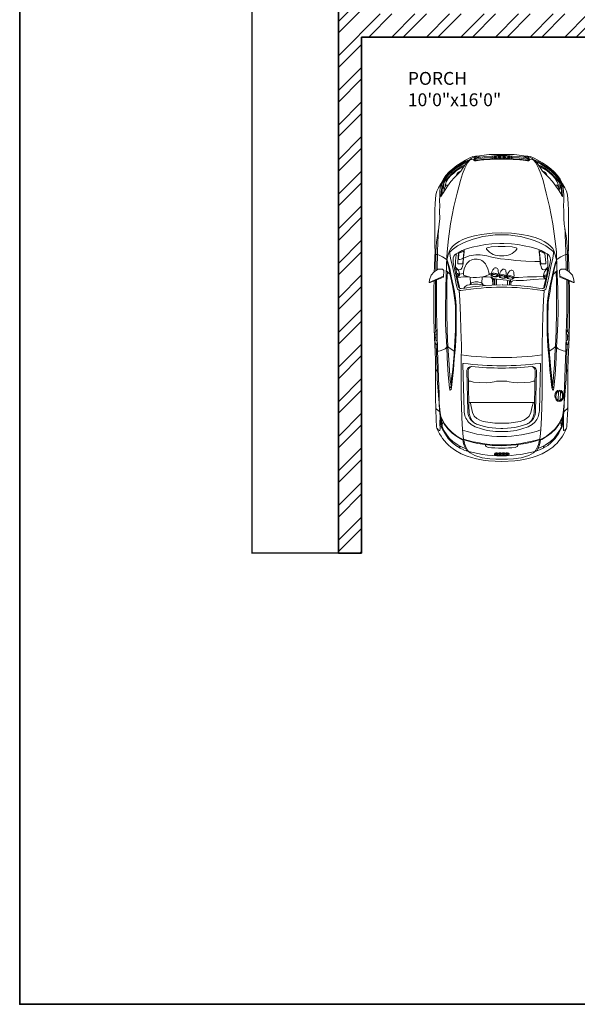
# Model space of a CAD drawing. Units: inches. Extents: x 1152 to 2588, y 1459 to 2618.
# Tile 1 of 17: x 1152 to 1369, y 1459 to 1843. Entities that reach past the tile are written whole.
import ezdxf

# ---------------------------------------------------------------- set-up
doc = ezdxf.new("R2010")
doc.units = ezdxf.units.IN
for name, color, linetype, lineweight in [('A-ANNO-DIMS', 2, 'Continuous', 18), ('A-ANNO-TTLB', 7, 'Continuous', 35), ('A-AREA-IDEN', 7, 'Continuous', 18), ('A-WALL', 7, 'Continuous', 35), ('A-WALL-PATT', 8, 'Continuous', 13), ('AUDI', 7, 'Continuous', 13)]:
    doc.layers.add(name, color=color, linetype=linetype, lineweight=lineweight)
doc.styles.get("Standard").update_dxf_attribs({"font": 'arial.ttf'})
doc.dimstyles.get("Standard").update_dxf_attribs({"dimtxt": 0.18, "dimasz": 0.18, "dimexe": 0.18, "dimexo": 0.0625, "dimgap": 0.09, "dimtad": 0, "dimtih": 1, "dimtoh": 1, "dimdec": 4, "dimzin": 0, "dimdsep": 46, "dimtxsty": 'Standard', "dimcen": 0.09, "dimadec": 0, "dimazin": 0, "dimtfac": 1, "dimtdec": 4, "dimtofl": 0, "dimtmove": 0, "dimatfit": 3, "dimfxl": 1, "dimtolj": 1, "dimtzin": 0, "dimarcsym": 0})

# ---------------------------------------------------------------- blocks, each defined once
blk = doc.blocks.new('*D71')
at = {"layer": 'A-ANNO-DIMS', "color": 0, "lineweight": -2, "transparency": 16777216}
for p, q in [((1276.35, 2240.05), (1242.64, 2240.05)), ((1242.82, 2239.87), (1242.82, 1937.73)), ((1242.82, 1635.23), (1242.82, 1937.36)), ((1276.35, 1635.05), (1242.64, 1635.05))]:
    blk.add_line(p, q, dxfattribs=at)
at = {"layer": 'A-ANNO-DIMS', "color": 0, "transparency": 16777216}
for points in [[(1242.79, 2239.87), (1242.85, 2239.87), (1242.82, 2240.05)], [(1242.79, 1635.23), (1242.85, 1635.23), (1242.82, 1635.05)]]:
    blk.add_solid(points, dxfattribs=at)
at = {"layer": 'Defpoints', "color": 0, "transparency": 16777216}
for p in [(1242.82, 2240.05), (1276.42, 2240.05), (1276.42, 1635.05)]:
    blk.add_point(p, dxfattribs=at)
at = {"layer": 'A-ANNO-DIMS', "color": 0, "transparency": 16777216, "insert": (1242.82, 1937.55), "char_height": 0.18, "attachment_point": 5}
blk.add_mtext('\\A1;605', dxfattribs=at)

msp = doc.modelspace()

# ---------------------------------------------------------------- hatches: boundary and pattern name
at = {"layer": 'A-WALL-PATT'}
h = msp.add_hatch(dxfattribs=at)
h.set_pattern_fill('ANSI32', color=256)
h.paths.add_polyline_path([(1408.9272, 2240.0458), (1276.4165, 2240.0458), (1276.4165, 2192.7491), (1285.4165, 2192.7491), (1285.4165, 2231.0458), (1369.4165, 2231.0458), (1369.4165, 2084.0458), (1526.9165, 2084.0458), (1526.9165, 2096.3728), (1524.6665, 2096.3728), (1522.4165, 2096.3728), (1522.4165, 2093.0458), (1378.4165, 2093.0458), (1378.4165, 2231.0458), (1408.9272, 2231.0458)])
h.paths.add_polyline_path([(1736.4165, 2240.0458), (1468.9272, 2240.0458), (1468.9272, 2231.0458), (1522.4165, 2231.0458), (1522.4165, 2127.3313), (1526.9165, 2127.3313), (1526.9165, 2231.0458), (1574.9165, 2231.0458), (1574.9165, 2188.0458), (1579.4165, 2188.0458), (1579.4165, 2231.0458), (1727.4165, 2231.0458), (1727.4165, 2183.9728), (1736.4165, 2183.9728)])
h.paths.add_polyline_path([(1285.4165, 2156.7491), (1276.4165, 2156.7491), (1276.4165, 2084.0458), (1285.4165, 2084.0458)], flags=17)
h.paths.add_polyline_path([(1285.4165, 2043.5458), (1445.4165, 2043.5458), (1445.4165, 1943.6503), (1454.4165, 1943.6503), (1454.4165, 2048.0458), (1276.4165, 2048.0458), (1276.4165, 2019.2077), (1280.9165, 2019.2077), (1285.4165, 2019.2077)])
h.paths.add_polyline_path([(1285.4165, 1959.2077), (1276.4165, 1959.2077), (1276.4165, 1891.1319), (1280.9165, 1891.1319), (1285.4165, 1891.1319), (1285.4165, 1901.0458), (1376.8505, 1901.0458), (1376.8505, 1903.2958), (1376.8505, 1905.5458), (1285.4165, 1905.5458)])
h.paths.add_polyline_path([(1518.4165, 1905.5458), (1399.2832, 1905.5458), (1399.2832, 1903.2958), (1399.2832, 1901.0458), (1405.4165, 1901.0458), (1405.4165, 1884.8579), (1409.9165, 1884.8579), (1409.9165, 1901.0458), (1513.9165, 1901.0458), (1513.9165, 1869.1706), (1518.4165, 1869.1706)])
h.paths.add_polyline_path([(1520.5229, 1845.0458), (1518.4165, 1845.0458), (1518.4165, 1849.2927), (1516.1665, 1849.2927), (1513.9165, 1849.2927), (1513.9165, 1845.0458), (1409.9165, 1845.0458), (1409.9165, 1860.8579), (1405.4165, 1860.8579), (1405.4165, 1845.0458), (1285.4165, 1845.0458), (1285.4165, 1867.1319), (1276.4165, 1867.1319), (1276.4165, 1635.0458), (1285.4165, 1635.0458), (1285.4165, 1836.0458), (1405.4165, 1836.0458), (1405.4165, 1635.0458), (1414.4165, 1635.0458), (1424.7277, 1635.0458), (1424.7277, 1639.5458), (1424.7277, 1644.0458), (1414.4165, 1644.0458), (1414.4165, 1836.0458), (1414.4165, 1840.5831), (1520.5229, 1840.5831)])
h.paths.add_polyline_path([(1579.4165, 1840.5458), (1583.4035, 1840.5458), (1583.4035, 1845.0458), (1579.4165, 1845.0458), (1570.4165, 1845.0458), (1570.4165, 1840.5831), (1570.4165, 1644.0458), (1548.2359, 1644.0458), (1548.2359, 1635.0458), (1611.2801, 1635.0458), (1611.2801, 1639.5458), (1611.2801, 1644.0458), (1579.4165, 1644.0458)])
h.paths.add_polyline_path([(1488.2359, 1644.0458), (1472.0663, 1644.0458), (1472.0663, 1635.0458), (1488.2359, 1635.0458), (1488.2359, 1639.5458)], flags=17)
h.paths.add_polyline_path([(1736.4165, 1701.1863), (1727.4165, 1701.1863), (1727.4165, 1644.0458), (1671.2801, 1644.0458), (1671.2801, 1635.0458), (1736.4165, 1635.0458)])
h.paths.add_polyline_path([(1736.4165, 2147.9728), (1727.4165, 2147.9728), (1727.4165, 2093.0458), (1579.4165, 2093.0458), (1574.9165, 2093.0458), (1574.9165, 1971.6501), (1579.4165, 1971.6501), (1579.4165, 2084.0458), (1727.4165, 2084.0458), (1727.4165, 2054.3847), (1736.4165, 2054.3847)])
h.paths.add_polyline_path([(1736.4165, 1994.3847), (1727.4165, 1994.3847), (1727.4165, 1911.3562), (1736.4165, 1911.3562)])
h.paths.add_polyline_path([(1736.4165, 1875.3562), (1727.4165, 1875.3562), (1727.4165, 1845.0458), (1617.1767, 1845.0458), (1617.1767, 1842.7958), (1617.1767, 1840.5458), (1618.9165, 1840.5458), (1618.9165, 1788.5458), (1618.9165, 1784.0458), (1627.8699, 1784.0458), (1627.8699, 1788.5458), (1623.4165, 1788.5458), (1623.4165, 1840.5458), (1727.4165, 1840.5458), (1727.4165, 1828.7619), (1736.4165, 1828.7619)])
h.paths.add_polyline_path([(1727.4165, 1938.0458), (1579.4165, 1938.0458), (1579.4165, 1942.7722), (1574.9165, 1942.7722), (1574.9165, 1929.0458), (1727.4165, 1929.0458)])

# ---------------------------------------------------------------- linework, layer by layer
at = {"layer": 'A-ANNO-TTLB'}
msp.add_lwpolyline([(1152.3215, 2617.6685), (2587.6987, 2617.6685), (2587.6987, 1459.3148), (1152.3215, 1459.3148)], close=True, dxfattribs=at)
at = {"layer": 'A-WALL'}
for p, q in [((1276.4165, 2048.0458), (1276.4165, 1635.0458)), ((1285.4165, 1836.0458), (1405.4165, 1836.0458)), ((1285.4165, 1836.0458), (1285.4165, 1635.0458)), ((1276.4165, 1635.0458), (1285.4165, 1635.0458))]:
    msp.add_line(p, q, dxfattribs=at)
at = {"layer": 'AUDI'}
for p, q in [((1336.2642, 1788.9641), (1336.2642, 1789.3086)), ((1338.3183, 1788.6147), (1338.3183, 1788.9592)), ((1341.9032, 1788.6147), (1341.9032, 1788.9592)), ((1343.9573, 1788.9641), (1343.9573, 1789.3086)), ((1324.4285, 1743.7759), (1323.5691, 1743.6789)), ((1325.138, 1743.8957), (1324.4285, 1743.7759)), ((1336.3949, 1741.7306), (1336.6785, 1741.7306)), ((1337.9694, 1741.854), (1337.9694, 1739.4675)), ((1342.3316, 1741.2324), (1342.3316, 1739.4615)), ((1352.8881, 1693.669), (1327.1848, 1693.669)), ((1323.4445, 1676.9323), (1323.6352, 1676.0919)), ((1323.8057, 1676.7406), (1323.7884, 1676.0051)), ((1356.2671, 1676.7406), (1356.2844, 1676.0051)), ((1356.6283, 1676.9323), (1356.4377, 1676.0919)), ((1337.1736, 1673.7524), (1337.1736, 1673.4961)), ((1338.7024, 1674.0125), (1338.7024, 1673.7561)), ((1341.3704, 1674.0125), (1341.3704, 1673.7561)), ((1342.8992, 1673.7524), (1342.8992, 1673.4961))]:
    msp.add_line(p, q, dxfattribs=at)
for points in [[(1330.6512, 1789.6915), (1329.8192, 1789.6915), (1328.8394, 1789.5322), (1327.6534, 1789.0235), (1325.9309, 1788.1193), (1324.2084, 1787.0173), (1322.5424, 1786.0283), (1320.9611, 1784.785), (1319.5492, 1783.5135), (1318.3056, 1782.1062), (1317.333, 1780.676), (1316.3603, 1778.928), (1315.4075, 1777.2992), (1314.7921, 1776.0477), (1314.4348, 1774.6573), (1314.1379, 1771.2484), (1314.0524, 1768.6062), (1314.0524, 1754.0739), (1314.0871, 1753.1593), (1314.1886, 1752.2446), (1313.9855, 1750.7203), (1313.8332, 1746.452), (1313.7887, 1744.543)], [(1314.0607, 1751.2847), (1314.4242, 1751.3887), (1315.0168, 1751.3145), (1315.6464, 1751.0551), (1317.0168, 1750.4251), (1318.4242, 1749.4985), (1318.7575, 1749.1279), (1319.1139, 1748.3445), (1319.7923, 1745.7397), (1320.518, 1742.235), (1321.3068, 1738.7145), (1321.6223, 1736.9622), (1321.7643, 1735.9518), (1322.0424, 1734.2928), (1322.3397, 1731.511), (1322.2994, 1728.038), (1322.3397, 1723.9593), (1322.2695, 1720.8795), (1322.0184, 1715.5567), (1321.5846, 1710.5309), (1321.2422, 1706.3732), (1320.8752, 1703.0862), (1320.4735, 1699.5786), (1320.2909, 1698.7748), (1319.9623, 1698.5556), (1319.8194, 1698.6697), (1319.6702, 1699.3959), (1319.1956, 1704.438), (1318.8305, 1711.0878), (1318.6844, 1715.3261), (1318.4288, 1719.674), (1318.2098, 1724.168), (1318.1002, 1729.6852), (1318.2165, 1737.9788), (1318.3917, 1743.4135), (1318.5669, 1747.2119), (1318.6399, 1750.1589), (1318.7567, 1752.3795), (1319.3407, 1757.522), (1320.1582, 1763.2488), (1321.443, 1770.0275), (1322.6693, 1775.2284), (1323.9541, 1780.1371), (1324.7793, 1782.7893), (1325.7137, 1785.0099), (1326.7064, 1787.0552), (1327.2327, 1787.7697), (1327.775, 1788.3646)], [(1329.2496, 1788.5039), (1328.2354, 1788.3227), (1327.2308, 1787.9457), (1326.603, 1787.5688), (1326.4356, 1787.3594), (1325.7241, 1786.1029), (1325.0126, 1785.1815), (1324.0918, 1783.8412), (1322.878, 1782.501), (1321.6642, 1781.412), (1320.1993, 1779.7786), (1318.9018, 1777.9357), (1317.981, 1776.5117), (1317.0602, 1775.1295), (1316.5998, 1774.1663), (1316.4324, 1773.9987), (1316.3487, 1773.9987), (1316.5161, 1775.7997), (1316.6835, 1777.5169), (1316.7254, 1778.6477), (1316.8091, 1779.1922), (1317.1858, 1779.9461), (1318.4414, 1781.789), (1319.6133, 1783.0035), (1320.9108, 1784.3438), (1322.2502, 1785.3071), (1324.1755, 1786.6055), (1325.8496, 1787.5269), (1327.3564, 1788.2808), (1327.775, 1788.3646), (1328.1516, 1788.7834), (1328.9469, 1789.1603), (1329.6584, 1789.4116), (1330.6167, 1789.67)], [(1326.4846, 1787.4206), (1324.8452, 1786.6055), (1323.3384, 1785.6422), (1321.9153, 1784.6788), (1320.7015, 1783.6737), (1319.5715, 1782.5847), (1318.7763, 1781.7471), (1318.0647, 1780.7419), (1317.3113, 1779.6948), (1317.0184, 1779.1503), (1316.782, 1779.016)], [(1340.0364, 1790.3413), (1340.0364, 1790.3413), (1337.6279, 1790.3413), (1337.6279, 1790.3413), (1335.1392, 1790.2551), (1332.1678, 1789.8744), (1330.6512, 1789.6915), (1330.3045, 1789.4748), (1329.878, 1789.215), (1329.3216, 1788.6539), (1329.1358, 1788.2666), (1329.2287, 1787.9292), (1329.5041, 1787.8441), (1330.0536, 1787.861), (1331.6987, 1788.1229), (1333.0121, 1788.2705), (1333.96, 1788.3095), (1335.5087, 1788.4025), (1338.0487, 1788.4335), (1339.9621, 1788.4335), (1340.0364, 1788.4335)], [(1331.9134, 1789.8437), (1331.2008, 1789.5527), (1330.4775, 1789.1907), (1329.8747, 1788.6679), (1329.5532, 1788.2658), (1329.4326, 1788.0044), (1329.4222, 1787.8694)], [(1329.6272, 1788.3584), (1330.854, 1788.5815), (1333.1941, 1788.9717), (1335.7508, 1789.1885), (1336.2748, 1789.2409)], [(1329.823, 1787.926), (1330.5526, 1788.0588), (1332.8927, 1788.4489), (1335.4494, 1788.6657), (1336.3669, 1788.7575)], [(1349.848, 1788.9716), (1349.1183, 1789.1043), (1346.7783, 1789.4945), (1344.2216, 1789.7112), (1342.0549, 1789.928), (1340.6682, 1789.9714), (1340.1107, 1789.9714), (1339.5533, 1789.9714), (1338.1666, 1789.928), (1335.9999, 1789.7112), (1333.4432, 1789.4945), (1331.1031, 1789.1043), (1330.1854, 1788.9374)], [(1340.0364, 1790.3413), (1340.0364, 1790.3413), (1342.4449, 1790.3413), (1342.4449, 1790.3413), (1344.9337, 1790.2551), (1347.905, 1789.8744), (1349.4217, 1789.6915), (1349.7683, 1789.4748), (1350.1949, 1789.215), (1350.7513, 1788.6539), (1350.937, 1788.2666), (1350.8441, 1787.9292), (1350.5688, 1787.8441), (1350.0192, 1787.861), (1348.3742, 1788.1229), (1347.0608, 1788.2705), (1346.1128, 1788.3095), (1344.5641, 1788.4025), (1342.0241, 1788.4335), (1340.1107, 1788.4335), (1340.0364, 1788.4335)], [(1340.1107, 1788.9905), (1340.1107, 1788.646)], [(1350.2499, 1787.926), (1349.5202, 1788.0588), (1347.1802, 1788.4489), (1344.6235, 1788.6657), (1343.8401, 1788.7441)], [(1350.4456, 1788.3584), (1349.2188, 1788.5815), (1346.8788, 1788.9717), (1344.3221, 1789.1885), (1343.9573, 1789.225)], [(1348.1595, 1789.8437), (1348.872, 1789.5527), (1349.5954, 1789.1907), (1350.1982, 1788.6679), (1350.5197, 1788.2658), (1350.6402, 1788.0044), (1350.6506, 1787.8694)], [(1349.4217, 1789.6915), (1350.2537, 1789.6915), (1351.2335, 1789.5322), (1352.4194, 1789.0235), (1354.1419, 1788.1193), (1355.8644, 1787.0173), (1357.5304, 1786.0283), (1359.1117, 1784.785), (1360.5236, 1783.5135), (1361.7672, 1782.1062), (1362.7399, 1780.676), (1363.7125, 1778.928), (1364.6653, 1777.2992), (1365.2807, 1776.0477), (1365.638, 1774.6573), (1365.935, 1771.2484), (1366.0204, 1768.6062), (1366.0204, 1754.0739), (1365.9858, 1753.1593), (1365.8842, 1752.2446), (1366.0873, 1750.7203), (1366.2396, 1746.452), (1366.2841, 1744.543)], [(1350.8232, 1788.5039), (1351.8375, 1788.3227), (1352.842, 1787.9457), (1353.4698, 1787.5688), (1353.6372, 1787.3594), (1354.3487, 1786.1029), (1355.0603, 1785.1815), (1355.9811, 1783.8412), (1357.1949, 1782.501), (1358.4086, 1781.412), (1359.8735, 1779.7786), (1361.171, 1777.9357), (1362.0918, 1776.5117), (1363.0126, 1775.1295), (1363.473, 1774.1663), (1363.6404, 1773.9987), (1363.7242, 1773.9987), (1363.5567, 1775.7997), (1363.3893, 1777.5169), (1363.3475, 1778.6477), (1363.2637, 1779.1922), (1362.8871, 1779.9461), (1361.6314, 1781.789), (1360.4595, 1783.0035), (1359.162, 1784.3438), (1357.8227, 1785.3071), (1355.8974, 1786.6055), (1354.2232, 1787.5269), (1352.7164, 1788.2808), (1352.2979, 1788.3646), (1351.9212, 1788.7834), (1351.126, 1789.1603), (1350.4144, 1789.4116), (1349.4562, 1789.67)], [(1366.0121, 1751.2847), (1365.6486, 1751.3887), (1365.056, 1751.3145), (1364.4264, 1751.0551), (1363.0561, 1750.4251), (1361.6487, 1749.4985), (1361.3153, 1749.1279), (1360.9589, 1748.3445), (1360.2805, 1745.7397), (1359.5548, 1742.235), (1358.766, 1738.7145), (1358.4505, 1736.9622), (1358.3085, 1735.9518), (1358.0305, 1734.2928), (1357.7331, 1731.511), (1357.7734, 1728.038), (1357.7331, 1723.9593), (1357.8033, 1720.8795), (1358.0545, 1715.5567), (1358.4882, 1710.5309), (1358.8306, 1706.3732), (1359.1977, 1703.0862), (1359.5993, 1699.5786), (1359.7819, 1698.7748), (1360.1105, 1698.5556), (1360.2534, 1698.6697), (1360.4026, 1699.3959), (1360.8772, 1704.438), (1361.2424, 1711.0878), (1361.3884, 1715.3261), (1361.644, 1719.674), (1361.8631, 1724.168), (1361.9726, 1729.6852), (1361.8563, 1737.9788), (1361.6811, 1743.4135), (1361.5059, 1747.2119), (1361.4329, 1750.1589), (1361.3161, 1752.3795), (1360.7321, 1757.522), (1359.9146, 1763.2488), (1358.6298, 1770.0275), (1357.4035, 1775.2284), (1356.1188, 1780.1371), (1355.2935, 1782.7893), (1354.3592, 1785.0099), (1353.3664, 1787.0552), (1352.8401, 1787.7697), (1352.2979, 1788.3646)], [(1353.5883, 1787.4206), (1355.2277, 1786.6055), (1356.7344, 1785.6422), (1358.1575, 1784.6788), (1359.3713, 1783.6737), (1360.5014, 1782.5847), (1361.2966, 1781.7471), (1362.0081, 1780.7419), (1362.7615, 1779.6948), (1363.0545, 1779.1503), (1363.2908, 1779.016)], [(1316.7036, 1774.3833), (1316.8091, 1775.9672), (1317.0184, 1777.6425), (1317.3113, 1778.8571), (1318.0229, 1779.988), (1319.3204, 1781.5376), (1320.4923, 1782.7941), (1321.4968, 1783.7156), (1322.292, 1784.3019), (1323.4221, 1785.0558), (1324.5522, 1785.7259), (1325.3055, 1786.061), (1325.8452, 1786.3168)], [(1317.9646, 1777.6641), (1318.1066, 1778.5639), (1318.4414, 1779.6948), (1319.1529, 1780.9094), (1320.3249, 1782.2497), (1321.3294, 1783.0873), (1322.4594, 1784.0506), (1323.7151, 1784.8464), (1324.8452, 1785.5584), (1325.4828, 1785.7904)], [(1363.3693, 1774.3833), (1363.2637, 1775.9672), (1363.0545, 1777.6425), (1362.7615, 1778.8571), (1362.05, 1779.988), (1360.7525, 1781.5376), (1359.5806, 1782.7941), (1358.5761, 1783.7156), (1357.7808, 1784.3019), (1356.6507, 1785.0558), (1355.5207, 1785.7259), (1354.7673, 1786.061), (1354.2276, 1786.3168)], [(1362.1082, 1777.6641), (1361.9662, 1778.5639), (1361.6314, 1779.6948), (1360.9199, 1780.9094), (1359.748, 1782.2497), (1358.7435, 1783.0873), (1357.6134, 1784.0506), (1356.3578, 1784.8464), (1355.2277, 1785.5584), (1354.59, 1785.7904)], [(1316.7942, 1779.0952), (1316.432, 1778.3862), (1316.1541, 1777.6679), (1316.0383, 1777.1813), (1315.9225, 1776.1154), (1315.8993, 1774.192), (1315.8762, 1772.2456), (1315.9457, 1770.4844), (1315.8762, 1768.0745), (1315.8993, 1765.4328), (1315.7372, 1763.2315), (1315.3667, 1760.8679), (1315.2761, 1758.8381), (1315.1279, 1755.7249), (1315.0909, 1752.6117), (1315.0168, 1750.9069), (1314.9057, 1746.6818), (1314.9057, 1745.3425)], [(1317.4377, 1779.058), (1317.395, 1777.3075), (1317.4355, 1776.9924), (1317.677, 1776.8005)], [(1317.5625, 1775.8834), (1317.7299, 1777.2237), (1318.0647, 1777.8519), (1318.3996, 1778.3546), (1318.9018, 1778.3964), (1319.2262, 1778.3964)], [(1362.5104, 1775.8834), (1362.3429, 1777.2237), (1362.0081, 1777.8519), (1361.6733, 1778.3546), (1361.171, 1778.3964), (1360.8467, 1778.3964)], [(1362.6351, 1779.058), (1362.6778, 1777.3075), (1362.6373, 1776.9924), (1362.3958, 1776.8005)], [(1363.2787, 1779.0952), (1363.6409, 1778.3862), (1363.9188, 1777.6679), (1364.0345, 1777.1813), (1364.1503, 1776.1154), (1364.1735, 1774.192), (1364.1966, 1772.2456), (1364.1272, 1770.4844), (1364.1966, 1768.0745), (1364.1735, 1765.4328), (1364.3356, 1763.2315), (1364.7061, 1760.8679), (1364.7968, 1758.8381), (1364.9449, 1755.7249), (1364.982, 1752.6117), (1365.056, 1750.9069), (1365.1671, 1746.6818), (1365.1671, 1745.3425)], [(1315.4252, 1761.2411), (1314.9798, 1758.6898), (1314.6464, 1756.3549), (1314.4983, 1754.2424), (1314.3872, 1752.4264), (1314.4242, 1750.7215), (1314.3501, 1747.7195), (1314.3501, 1744.9448)], [(1364.6476, 1761.2411), (1365.0931, 1758.6898), (1365.4264, 1756.3549), (1365.5745, 1754.2424), (1365.6856, 1752.4264), (1365.6486, 1750.7215), (1365.7227, 1747.7195), (1365.7227, 1744.9448)], [(1340.0364, 1759.7866), (1336.2592, 1759.6279), (1332.2282, 1759.2033), (1329.4277, 1758.6514), (1327.0091, 1757.972), (1324.9299, 1757.1652), (1323.5297, 1756.4859), (1322.0446, 1755.5517), (1321.0262, 1754.66), (1320.1776, 1753.6835), (1319.626, 1752.4946), (1319.4138, 1751.985), (1319.0744, 1750.8811), (1318.8198, 1749.6922), (1318.7253, 1749.1638)], [(1319.7479, 1752.2791), (1320.1695, 1752.6665), (1320.7363, 1753.1728), (1322.8111, 1754.6981), (1325.394, 1756.0116), (1327.0665, 1756.6684), (1328.9758, 1757.356), (1330.3985, 1757.7627), (1332.7358, 1758.3051), (1334.8021, 1758.6102), (1337.4267, 1758.9572), (1340.0364, 1758.9572)], [(1340.0364, 1759.7866), (1343.8136, 1759.6279), (1347.8446, 1759.2033), (1350.6451, 1758.6514), (1353.0637, 1757.972), (1355.1429, 1757.1652), (1356.5431, 1756.4859), (1358.0283, 1755.5517), (1359.0466, 1754.66), (1359.8953, 1753.6835), (1360.4469, 1752.4946), (1360.659, 1751.985), (1360.9985, 1750.8811), (1361.2531, 1749.6922), (1361.3476, 1749.1638)], [(1360.325, 1752.2791), (1359.9033, 1752.6665), (1359.3365, 1753.1728), (1357.2618, 1754.6981), (1354.6789, 1756.0116), (1353.0064, 1756.6684), (1351.097, 1757.356), (1349.6743, 1757.7627), (1347.337, 1758.3051), (1345.2707, 1758.6102), (1342.6461, 1758.9572), (1340.0364, 1758.9572)], [(1322.0302, 1746.3617), (1322.4827, 1745.9913), (1323.0154, 1745.5598), (1323.6242, 1745.4075), (1324.1061, 1745.5344), (1324.512, 1745.9913), (1324.715, 1746.7274), (1324.994, 1747.7428), (1325.2223, 1750.3827), (1325.4252, 1752.3118), (1325.4417, 1753.166)], [(1322.8885, 1747.7428), (1324.7657, 1747.7428), (1324.8418, 1747.9459), (1325.0447, 1749.3927), (1325.1716, 1751.0427), (1325.2984, 1752.1849), (1325.2984, 1752.5149), (1325.2223, 1752.6419), (1325.0194, 1752.5657), (1323.9539, 1752.1088), (1323.2183, 1751.728), (1323.0915, 1750.535), (1322.9139, 1748.2505), (1322.8885, 1747.7428)], [(1358.0426, 1746.3617), (1357.5902, 1745.9913), (1357.0575, 1745.5598), (1356.4487, 1745.4075), (1355.9667, 1745.5344), (1355.5608, 1745.9913), (1355.3579, 1746.7274), (1355.0788, 1747.7428), (1354.8505, 1750.3827), (1354.6476, 1752.3118), (1354.6312, 1753.166)], [(1357.1843, 1747.7428), (1355.3071, 1747.7428), (1355.231, 1747.9459), (1355.0281, 1749.3927), (1354.9013, 1751.0427), (1354.7744, 1752.1849), (1354.7744, 1752.5149), (1354.8505, 1752.6419), (1355.0535, 1752.5657), (1356.1189, 1752.1088), (1356.8545, 1751.728), (1356.9814, 1750.535), (1357.1589, 1748.2505), (1357.1843, 1747.7428)], [(1323.7178, 1738.1535), (1323.472, 1739.1377), (1322.9393, 1741.3207), (1322.6349, 1742.8945), (1322.2543, 1745.0775), (1322.026, 1746.1436), (1322.0514, 1747.4636), (1322.0768, 1748.8089), (1322.1529, 1750.0019), (1322.2543, 1751.0427), (1322.4154, 1751.6737)], [(1356.355, 1738.1535), (1356.6009, 1739.1377), (1357.1336, 1741.3207), (1357.438, 1742.8945), (1357.8185, 1745.0775), (1358.0468, 1746.1436), (1358.0214, 1747.4636), (1357.9961, 1748.8089), (1357.9199, 1750.0019), (1357.8185, 1751.0427), (1357.6575, 1751.6737)], [(1317.5417, 1745.1151), (1317.3984, 1742.576), (1312.1954, 1740.4633), (1311.7752, 1740.5105), (1311.8853, 1741.4918), (1312.5102, 1743.2669), (1313.7886, 1744.5429), (1315.3313, 1745.6471), (1316.9347, 1745.6772), (1317.5417, 1745.1151)], [(1318.4717, 1745.1488), (1319.0654, 1744.4359), (1319.728, 1743.806), (1319.9283, 1743.7169)], [(1318.6046, 1748.7346), (1319.1979, 1747.2208), (1319.5623, 1745.4637), (1319.993, 1743.4082), (1320.9206, 1739.2641), (1321.2188, 1737.0429), (1321.7158, 1734.4238), (1321.9145, 1732.6336), (1321.9808, 1730.8102), (1322.0471, 1728.3569), (1322.0605, 1726.0316), (1322.0239, 1721.8281), (1321.8242, 1717.5118), (1321.4647, 1712.436), (1320.9455, 1706.561), (1320.5461, 1703.004), (1320.3065, 1700.1664), (1320.1894, 1699.5616), (1320.1431, 1699.4714), (1320.0488, 1699.4369), (1319.9421, 1699.4976), (1319.9023, 1699.657), (1319.8863, 1699.9278)], [(1361.4682, 1748.7346), (1360.8749, 1747.2208), (1360.5105, 1745.4637), (1360.0798, 1743.4082), (1359.1522, 1739.2641), (1358.854, 1737.0429), (1358.3571, 1734.4238), (1358.1583, 1732.6336), (1358.092, 1730.8102), (1358.0258, 1728.3569), (1358.0123, 1726.0316), (1358.049, 1721.8281), (1358.2487, 1717.5118), (1358.6081, 1712.436), (1359.1273, 1706.561), (1359.5267, 1703.004), (1359.7663, 1700.1664), (1359.8834, 1699.5616), (1359.9298, 1699.4714), (1360.024, 1699.4369), (1360.1308, 1699.4976), (1360.1706, 1699.657), (1360.1865, 1699.9278)], [(1361.6011, 1745.1488), (1361.0075, 1744.4359), (1360.3449, 1743.806), (1360.1445, 1743.7169)], [(1362.5312, 1745.1151), (1362.6744, 1742.576), (1367.8774, 1740.4633), (1368.2977, 1740.5105), (1368.1875, 1741.4918), (1367.5626, 1743.2669), (1366.2842, 1744.5429), (1364.7415, 1745.6471), (1363.1381, 1745.6772), (1362.5312, 1745.1151)], [(1311.7752, 1740.5105), (1317.4158, 1742.8834)], [(1314.3186, 1721.5502), (1314.2681, 1723.0036), (1314.1933, 1733.4027), (1314.1933, 1741.2746)], [(1314.6498, 1741.4599), (1314.6498, 1734.4092), (1314.6498, 1728.7684), (1314.8738, 1720.5125), (1315.0604, 1713.8257), (1315.3114, 1707.1608), (1315.61, 1699.7492), (1315.6499, 1697.4763), (1315.7342, 1692.6745), (1316.0089, 1688.2914), (1316.0016, 1685.5126), (1316.0063, 1683.488)], [(1318.716, 1740.6042), (1318.8667, 1744.6744)], [(1322.7473, 1742.3133), (1324.1093, 1742.5579), (1325.1687, 1742.6358), (1327.1508, 1742.6313), (1327.3253, 1742.6331)], [(1325.1533, 1743.2694), (1327.1508, 1742.6313), (1327.3253, 1742.6331)], [(1327.7889, 1742.5488), (1327.8753, 1739.9336)], [(1332.4317, 1742.631), (1332.2827, 1740.1385)], [(1332.7005, 1742.6877), (1334.3699, 1742.7046), (1335.799, 1742.5579), (1336.3853, 1742.4479), (1336.6052, 1742.2646), (1336.6785, 1741.8979), (1336.6785, 1741.6412), (1337.0029, 1741.6412)], [(1335.0916, 1743.9219), (1335.9933, 1743.8091)], [(1335.1977, 1743.5138), (1335.9119, 1743.3634)], [(1335.8326, 1742.5516), (1336.3949, 1741.7306), (1336.5474, 1739.4305)], [(1336.983, 1741.9676), (1337.1367, 1739.4458)], [(1336.983, 1741.9676), (1338.3033, 1741.8155), (1339.6716, 1741.6579), (1340.6609, 1741.5111), (1341.8523, 1741.3082), (1342.8157, 1741.156), (1343.5001, 1741.0799)], [(1337.3706, 1741.9229), (1337.4012, 1739.4527)], [(1343.1233, 1741.1218), (1343.1025, 1739.4415)], [(1343.5255, 1741.3843), (1343.4241, 1740.9784), (1343.4241, 1740.5979), (1343.5255, 1740.5471), (1343.7536, 1740.5471), (1344.1085, 1740.9277), (1344.362, 1741.156), (1345.7014, 1741.2854), (1348.5812, 1741.2854), (1352.475, 1741.5696), (1356.5025, 1741.8596), (1357.2494, 1741.9194)], [(1356.2625, 1742.7802), (1353.5853, 1742.7132), (1350.0196, 1742.6127), (1346.5543, 1742.462), (1344.6459, 1742.4117)], [(1361.3568, 1740.6042), (1361.2061, 1744.6744)], [(1368.2977, 1740.5105), (1362.6571, 1742.8834)], [(1365.423, 1741.4599), (1365.423, 1734.4092), (1365.423, 1728.7684), (1365.1991, 1720.5125), (1365.0124, 1713.8257), (1364.7614, 1707.1608), (1364.4628, 1699.7492), (1364.4229, 1697.4763), (1364.3386, 1692.6745), (1364.0639, 1688.2914), (1364.0713, 1685.5126), (1364.0666, 1683.488)], [(1365.7542, 1721.5502), (1365.8047, 1723.0036), (1365.8795, 1733.4027), (1365.8795, 1741.2746)], [(1320.2929, 1700.0963), (1320.0535, 1701.5689), (1319.8834, 1704.0845), (1319.5168, 1708.4046), (1319.2928, 1712.1541), (1319.0688, 1715.496), (1318.7681, 1721.5778), (1318.664, 1728.9799), (1318.664, 1736.9032), (1318.716, 1740.6042)], [(1340.4542, 1739.5103), (1340.0364, 1739.5103)], [(1343.6117, 1740.5471), (1343.5436, 1739.43)], [(1359.7799, 1700.0963), (1360.0193, 1701.5689), (1360.1895, 1704.0845), (1360.556, 1708.4046), (1360.78, 1712.1541), (1361.004, 1715.496), (1361.3047, 1721.5778), (1361.4089, 1728.9799), (1361.4089, 1736.9032), (1361.3568, 1740.6042)], [(1314.4383, 1718.1045), (1314.3802, 1719.778)], [(1365.6345, 1718.1045), (1365.6927, 1719.778)], [(1316.3608, 1688.2507), (1316.041, 1689.6293), (1315.5982, 1694.8727), (1315.3276, 1698.2206), (1314.9339, 1702.7747), (1314.8384, 1706.5868), (1314.5008, 1716.3051)], [(1321.5586, 1713.7614), (1320.9465, 1714.1289), (1319.9521, 1714.7779), (1319.3035, 1715.3187), (1319.067, 1715.533), (1318.8063, 1715.4268), (1318.5685, 1715.0807), (1317.9847, 1714.6048), (1317.12, 1714.1721), (1316.1255, 1713.8044), (1315.4632, 1713.7165), (1315.0606, 1713.7589), (1314.9405, 1713.9781), (1314.7216, 1714.4163), (1314.555, 1714.7446)], [(1358.5143, 1713.7614), (1359.1263, 1714.1289), (1360.1208, 1714.7779), (1360.7694, 1715.3187), (1361.0059, 1715.533), (1361.2666, 1715.4268), (1361.5044, 1715.0807), (1362.0881, 1714.6048), (1362.9529, 1714.1721), (1363.9473, 1713.8044), (1364.6096, 1713.7165), (1365.0122, 1713.7589), (1365.1323, 1713.9781), (1365.3513, 1714.4163), (1365.5178, 1714.7446)], [(1363.712, 1688.2507), (1364.0319, 1689.6293), (1364.4747, 1694.8727), (1364.7453, 1698.2206), (1365.1389, 1702.7747), (1365.2344, 1706.5868), (1365.572, 1716.3051)], [(1314.8384, 1706.5877), (1314.5608, 1706.2216), (1314.2996, 1705.5757)], [(1365.2344, 1706.5877), (1365.512, 1706.2216), (1365.7732, 1705.5757)], [(1327.0679, 1701.9611), (1327.8457, 1701.9611), (1328.9905, 1701.6404), (1331.3258, 1701.4571), (1333.9358, 1701.4113), (1335.4927, 1701.5488), (1337.1412, 1701.732), (1338.0112, 1701.9611), (1340.0364, 1701.9611)], [(1353.0049, 1701.9611), (1352.2271, 1701.9611), (1351.0824, 1701.6404), (1348.747, 1701.4571), (1346.137, 1701.4113), (1344.5801, 1701.5488), (1342.9316, 1701.732), (1342.0616, 1701.9611), (1340.0364, 1701.9611)], [(1362.1465, 1698.0896), (1362.0837, 1694.5434)], [(1362.9115, 1698.0381), (1362.8501, 1694.5708)], [(1314.3236, 1691.6391), (1314.6633, 1691.1801), (1315.1553, 1690.7862), (1315.8955, 1690.1012)], [(1332.8174, 1686.3346), (1331.4737, 1686.8379), (1330.3987, 1687.4296), (1329.2969, 1688.3439), (1328.7056, 1689.7961), (1328.1413, 1692.1088), (1327.8456, 1693.4535)], [(1347.2554, 1686.3346), (1348.5991, 1686.8379), (1349.6741, 1687.4296), (1350.776, 1688.3439), (1351.3672, 1689.7961), (1351.9316, 1692.1088), (1352.2272, 1693.4535)], [(1365.7493, 1691.6391), (1365.4095, 1691.1801), (1364.9175, 1690.7862), (1364.1773, 1690.1012)], [(1325.258, 1675.2256), (1323.9095, 1675.9365), (1322.1097, 1676.9559), (1320.7175, 1678.1452), (1319.2234, 1679.6743), (1317.8311, 1681.7471), (1316.9821, 1683.3101), (1316.5067, 1684.2616), (1316.303, 1685.315), (1316.303, 1686.6402), (1316.269, 1688.1353), (1316.2475, 1688.7391)], [(1324.8756, 1679.1312), (1324.4672, 1679.3457), (1322.5433, 1680.4172), (1320.7103, 1681.7975), (1319.1313, 1683.3412), (1317.7848, 1685.2026), (1316.6523, 1687.411), (1316.2665, 1688.2076)], [(1325.258, 1679.1682), (1324.4672, 1679.5836), (1322.5433, 1680.6551), (1320.7103, 1682.0353), (1319.1313, 1683.5791), (1317.7848, 1685.4405), (1316.6523, 1687.6489), (1316.3608, 1688.2507)], [(1325.9558, 1675.7657), (1324.9237, 1676.1474), (1323.0737, 1677.1291), (1320.9714, 1678.5315), (1319.626, 1679.8779), (1318.3926, 1681.4486), (1317.5237, 1682.851), (1317.0472, 1683.7206), (1316.7949, 1684.3657), (1316.6828, 1685.1791), (1316.5987, 1686.5255), (1316.5987, 1687.5217)], [(1354.117, 1675.7657), (1355.1491, 1676.1474), (1356.9991, 1677.1291), (1359.1014, 1678.5315), (1360.4469, 1679.8779), (1361.6802, 1681.4486), (1362.5492, 1682.851), (1363.0257, 1683.7206), (1363.2779, 1684.3657), (1363.3901, 1685.1791), (1363.4741, 1686.5255), (1363.4741, 1687.5217)], [(1354.8148, 1675.2256), (1356.1633, 1675.9365), (1357.9631, 1676.9559), (1359.3554, 1678.1452), (1360.8495, 1679.6743), (1362.2417, 1681.7471), (1363.0907, 1683.3101), (1363.5661, 1684.2616), (1363.7698, 1685.315), (1363.7698, 1686.6402), (1363.8038, 1688.1353), (1363.8253, 1688.7391)], [(1354.8148, 1679.1682), (1355.6056, 1679.5836), (1357.5295, 1680.6551), (1359.3626, 1682.0353), (1360.9415, 1683.5791), (1362.288, 1685.4405), (1363.4205, 1687.6489), (1363.712, 1688.2507)], [(1355.1972, 1679.1312), (1355.6056, 1679.3457), (1357.5295, 1680.4172), (1359.3626, 1681.7975), (1360.9415, 1683.3412), (1362.288, 1685.2026), (1363.4205, 1687.411), (1363.8064, 1688.2076)], [(1316.0063, 1683.488), (1316.0003, 1682.9865), (1315.8773, 1682.8326), (1315.6467, 1682.8326), (1315.4622, 1682.9096), (1315.2623, 1683.1096), (1314.9855, 1683.4327), (1314.8044, 1683.6551)], [(1317.409, 1686.1734), (1317.1313, 1685.7962), (1316.907, 1685.4035), (1316.8229, 1684.8425), (1316.7949, 1684.0572), (1316.8348, 1683.6051)], [(1362.6638, 1686.1734), (1362.9416, 1685.7962), (1363.1658, 1685.4035), (1363.2499, 1684.8425), (1363.2779, 1684.0572), (1363.2381, 1683.6051)], [(1364.0666, 1683.488), (1364.0725, 1682.9865), (1364.1955, 1682.8326), (1364.4262, 1682.8326), (1364.6107, 1682.9096), (1364.8105, 1683.1096), (1365.0873, 1683.4327), (1365.2684, 1683.6551)], [(1326.4196, 1674.8747), (1326.0149, 1675.6307), (1325.3018, 1677.2617), (1325.0301, 1678.451), (1324.8756, 1679.1312)], [(1334.7921, 1676.2104), (1334.0284, 1676.5329), (1333.7019, 1676.9412), (1333.601, 1677.3046)], [(1345.3054, 1676.2208), (1346.0445, 1676.5329), (1346.3709, 1676.9412), (1346.4743, 1677.3136)], [(1353.6532, 1674.8747), (1354.058, 1675.6307), (1354.7711, 1677.2617), (1355.0427, 1678.451), (1355.1972, 1679.1312)], [(1340.0364, 1673.7329), (1340.0364, 1673.9892)]]:
    msp.add_lwpolyline(points, dxfattribs=at)
for points in [[(1322.3041, 1781.9861, -0.27931409), (1324.0506, 1783.7958, -0.27931409)], [(1357.7687, 1781.9861, 0.27931409), (1356.0222, 1783.7958, 0.27931409)], [(1319.6901, 1752.6328), (1320.1348, 1749.9102), (1320.8443, 1746.6447), (1321.731, 1742.5983), (1322.334, 1739.8653), (1322.6888, 1738.339, 0.36424732), (1324.1076, 1737.2742, -0.04353666), (1340.0364, 1738.6514)], [(1340.0364, 1755.5947), (1339.2695, 1755.5947), (1336.2344, 1755.4862), (1333.7413, 1755.2151), (1331.3023, 1754.7812), (1328.5779, 1754.1919), (1326.3816, 1753.5242), (1324.63, 1752.8565), (1323.0731, 1752.0497), (1322.2946, 1751.6046), (1321.7941, 1751.2429), (1321.3771, 1750.6865), (1321.1825, 1750.0466), (1321.0713, 1749.3233), (1321.0991, 1748.2939), (1323.2121, 1738.7514, 0.41343093), (1324.213, 1738.1115), (1325.6952, 1738.3085), (1328.72, 1738.7981), (1332.6346, 1739.1987), (1336.1933, 1739.4213), (1339.6186, 1739.5103)], [(1340.0364, 1754.4399), (1338.6805, 1754.4399), (1335.9733, 1754.2935), (1334.9932, 1754.0893), (1334.3979, 1753.9636), (1334.1745, 1753.8071), (1334.1075, 1753.6506), (1334.1522, 1753.4606, 0.25546602), (1340.0364, 1750.8445, 2.79521639)], [(1340.0364, 1755.5947), (1340.8034, 1755.5947), (1343.8385, 1755.4862), (1346.3316, 1755.2151), (1348.7705, 1754.7812), (1351.4949, 1754.1919), (1353.6913, 1753.5242), (1355.4428, 1752.8565), (1356.9998, 1752.0497), (1357.7782, 1751.6046), (1358.2787, 1751.2429), (1358.6957, 1750.6865), (1358.8904, 1750.0466), (1359.0016, 1749.3233), (1358.9738, 1748.2939), (1356.8608, 1738.7514, -0.41343093), (1355.8599, 1738.1115), (1354.3777, 1738.3085), (1351.3528, 1738.7981), (1347.4382, 1739.1987), (1343.8795, 1739.4213), (1340.4542, 1739.5103)], [(1340.0364, 1754.4399), (1341.3923, 1754.4399), (1344.0995, 1754.2935), (1345.0796, 1754.0893), (1345.6749, 1753.9636), (1345.8983, 1753.8071), (1345.9653, 1753.6506), (1345.9206, 1753.4606, -0.25546602), (1340.0364, 1750.8445, -2.79521639)], [(1360.3827, 1752.6328), (1359.938, 1749.9102), (1359.2286, 1746.6447), (1358.3418, 1742.5983), (1357.7388, 1739.8653), (1357.3841, 1738.339, -0.36424732), (1355.9653, 1737.2742, 0.04353666), (1340.0364, 1738.6514)], [(1355.005, 1748.5972), (1352.9395, 1748.5972), (1349.4221, 1748.7409), (1345.474, 1749.0282), (1342.8181, 1749.4592), (1339.516, 1749.6747), (1336.214, 1750.3212), (1334.2758, 1750.824, 0.12760018), (1327.3128, 1750.824), (1325.7601, 1750.2196), (1324.9684, 1749.8801), (1324.2144, 1749.5594), (1323.7243, 1749.4651), (1323.4039, 1749.4651), (1323.2719, 1749.7858), (1323.3569, 1751.3091)], [(1335.1977, 1743.5138), (1335.0756, 1744.4609), (1334.6787, 1745.8356), (1334.007, 1747.2409, 0.61645483), (1325.9471, 1746.966), (1325.4281, 1745.8051), (1325.1228, 1744.522), (1325.1533, 1743.2694, 0.20084491), (1335.1977, 1743.5138, 3.44889889)], [(1322.2203, 1745.2363, -0.43942644), (1322.9173, 1745.3978), (1323.1999, 1745.0714), (1323.4382, 1744.4918), (1323.5433, 1743.8704), (1323.6102, 1743.3751), (1323.6035, 1743.207), (1323.4208, 1742.9282, -0.09128884), (1322.6674, 1742.7261, -0.09128884)], [(1338.6754, 1743.2023), (1338.71, 1743.6178), (1338.7273, 1744.1719), (1338.71, 1744.7953), (1338.6235, 1745.4187, 0.69697601), (1336.9622, 1745.7824), (1336.6161, 1745.3495), (1336.2181, 1744.6222), (1336.045, 1744.0161), (1335.9239, 1743.5312), (1335.9119, 1743.3634), (1336.2354, 1742.9425, 0.1146222), (1338.1389, 1742.7174), (1338.3812, 1742.8213), (1338.6061, 1742.9945), (1338.6754, 1743.2023)], [(1341.7598, 1742.6597), (1341.7944, 1743.0753), (1341.8117, 1743.6294), (1341.7944, 1744.2528), (1341.7079, 1744.8761, 0.69697601), (1340.0466, 1745.2398), (1339.7005, 1744.8069), (1339.3025, 1744.0796), (1339.1295, 1743.4735), (1339.0083, 1742.9887), (1338.9963, 1742.8208), (1339.3198, 1742.3999, 0.1146222), (1341.2233, 1742.1748), (1341.4656, 1742.2787), (1341.6906, 1742.4519), (1341.7598, 1742.6597)], [(1344.7813, 1742.2378), (1344.8159, 1742.6534), (1344.8332, 1743.2075), (1344.8159, 1743.8309), (1344.7294, 1744.4543, 0.69697601), (1343.0681, 1744.8179), (1342.722, 1744.385), (1342.324, 1743.6577), (1342.151, 1743.0517), (1342.0298, 1742.5668), (1342.0178, 1742.399), (1342.3413, 1741.978, 0.1146222), (1344.2448, 1741.7529), (1344.4871, 1741.8568), (1344.7121, 1742.03), (1344.7813, 1742.2378)], [(1357.9249, 1745.5744, 0.30781353), (1357.0379, 1745.0722), (1356.7417, 1744.6037), (1356.4264, 1743.8369), (1356.3213, 1743.2155), (1356.2544, 1742.7202), (1356.261, 1742.5521), (1356.4438, 1742.2733, 0.10075057), (1357.2778, 1742.0662, 0.03883263)], [(1313.708, 1741.0775), (1313.641, 1738.2022), (1313.641, 1726.0932), (1313.8034, 1719.0228), (1314.2095, 1710.4083), (1314.2996, 1706.678), (1314.2996, 1703.2946), (1314.2244, 1695.4751), (1314.3371, 1691.1142), (1314.4874, 1686.9413), (1314.6377, 1684.4225), (1314.8255, 1683.5578, 0.12683503), (1320.1669, 1676.3808), (1322.0897, 1674.9979), (1324.2528, 1673.7352), (1326.5961, 1672.7732), (1328.2185, 1672.2922), (1330.2013, 1671.751), (1332.8451, 1671.27), (1334.9481, 1670.9694), (1340.0364, 1670.7948)], [(1323.5035, 1737.7063), (1323.7382, 1733.6354), (1324.0512, 1727.5681), (1324.0903, 1722.088), (1324.325, 1715.9033), (1324.2468, 1709.6795), (1324.2586, 1696.6997), (1324.4802, 1687.7858), (1324.7543, 1683.206), (1325.0558, 1680.3264), (1325.2714, 1679.0918, 0.10917638), (1327.1131, 1674.6162), (1327.6954, 1674.075), (1329.5309, 1673.1304), (1332.4677, 1672.212), (1335.457, 1671.766), (1337.7382, 1671.661), (1340.0364, 1671.661)], [(1323.5229, 1737.3695), (1323.7382, 1733.6354), (1324.0512, 1727.5681), (1324.0903, 1722.088), (1324.325, 1715.9033), (1324.2468, 1709.6795), (1324.2586, 1696.6997), (1324.4802, 1687.7858), (1324.7543, 1683.206), (1325.0558, 1680.3264), (1325.2714, 1679.0918, 0.10917638), (1327.1131, 1674.6162), (1327.6954, 1674.075), (1329.5309, 1673.1304), (1332.4677, 1672.212), (1335.457, 1671.766), (1337.7382, 1671.661), (1340.0364, 1671.661)], [(1333.6811, 1739.2642), (1333.2457, 1739.4578, 0.09257149), (1326.6168, 1739.4578), (1325.8504, 1738.921), (1325.261, 1738.2508)], [(1330.2001, 1740.7048, 0.11496238), (1328.2644, 1740.263), (1327.7663, 1739.8412), (1327.7051, 1739.6269)], [(1330.2001, 1740.7048, -0.11496238), (1332.1357, 1740.263), (1332.6338, 1739.8412), (1332.7174, 1739.5484)], [(1366.3648, 1741.0775), (1366.4318, 1738.2022), (1366.4318, 1726.0932), (1366.2694, 1719.0228), (1365.8633, 1710.4083), (1365.7732, 1706.678), (1365.7732, 1703.2946), (1365.8484, 1695.4751), (1365.7357, 1691.1142), (1365.5854, 1686.9413), (1365.4351, 1684.4225), (1365.2473, 1683.5578, -0.12683503), (1359.9059, 1676.3808), (1357.9832, 1674.9979), (1355.8201, 1673.7352), (1353.4767, 1672.7732), (1351.8544, 1672.2922), (1349.8715, 1671.751), (1347.2277, 1671.27), (1345.1247, 1670.9694), (1340.0364, 1670.7948)], [(1356.5499, 1737.3695), (1356.3346, 1733.6354), (1356.0217, 1727.5681), (1355.9825, 1722.088), (1355.7478, 1715.9033), (1355.8261, 1709.6795), (1355.8142, 1696.6997), (1355.5926, 1687.7858), (1355.3185, 1683.206), (1355.0171, 1680.3264), (1354.8015, 1679.0918, -0.10917638), (1352.9598, 1674.6162), (1352.3775, 1674.075), (1350.5419, 1673.1304), (1347.6051, 1672.212), (1344.6159, 1671.766), (1342.3346, 1671.661), (1340.0364, 1671.661)], [(1314.7264, 1721.8311), (1314.8179, 1720.3675), (1314.8179, 1720.3675), (1314.6613, 1720.3782), (1314.5394, 1720.2867), (1314.448, 1720.0122, 0.17711693), (1314.5089, 1717.9083), (1314.636, 1717.8066), (1314.8016, 1717.7097), (1314.8016, 1717.7097), (1314.8788, 1717.6537), (1314.8483, 1716.8914), (1314.7569, 1716.251), (1314.4175, 1716.3227), (1314.3313, 1716.4974, -0.20734628), (1314.3618, 1721.6506), (1314.387, 1721.7198), (1314.6004, 1721.8723), (1314.7264, 1721.8311)], [(1365.3464, 1721.8311), (1365.255, 1720.3675), (1365.255, 1720.3675), (1365.4115, 1720.3782), (1365.5334, 1720.2867), (1365.6249, 1720.0122, -0.17711693), (1365.5639, 1717.9083), (1365.4369, 1717.8066), (1365.2712, 1717.7097), (1365.2712, 1717.7097), (1365.194, 1717.6537), (1365.2245, 1716.8914), (1365.3159, 1716.251), (1365.6553, 1716.3227), (1365.7415, 1716.4974, 0.20734628), (1365.711, 1721.6506), (1365.6858, 1721.7198), (1365.4725, 1721.8723), (1365.3464, 1721.8311)], [(1355.7939, 1712.2383, -0.06516086), (1324.2789, 1712.2365, -4.49164968)], [(1325.1421, 1708.9547, 0.4622712), (1324.9347, 1708.698), (1325.3772, 1690.501, 0.18047602), (1327.1422, 1686.1001), (1328.126, 1685.1736), (1329.7463, 1684.1891), (1332.1479, 1683.4363), (1334.3469, 1682.7994), (1337.6508, 1682.4147), (1340.0364, 1682.4147)], [(1354.9307, 1708.9547, -0.0615843), (1325.1321, 1708.9542, -0.0615843)], [(1328.2257, 1707.6959, 0.40402709), (1326.5133, 1706.2121), (1326.8214, 1690.3035, 0.22167644), (1328.8441, 1686.1759, 0.05999808), (1330.2035, 1685.3256), (1332.7972, 1684.4507), (1334.9247, 1684.0133), (1337.7806, 1683.6925), (1339.6458, 1683.6342), (1340.0364, 1683.6342)], [(1329.2954, 1685.8421, -0.17077992), (1327.3767, 1689.4957), (1327.2018, 1692.5286), (1327.0853, 1700.3148), (1327.0251, 1706.0196, -0.32699174), (1328.2257, 1707.6959, -1.80630344)], [(1351.8471, 1707.6959, -0.04880378), (1328.1993, 1707.6971, -0.04880378)], [(1354.9307, 1708.9547, -0.4622712), (1355.1381, 1708.698), (1354.6956, 1690.501, -0.18047602), (1352.9306, 1686.1001), (1351.9469, 1685.1736), (1350.3265, 1684.1891), (1347.9249, 1683.4363), (1345.7259, 1682.7994), (1342.4221, 1682.4147), (1340.0364, 1682.4147)], [(1351.8471, 1707.6959, -0.40402709), (1353.5596, 1706.2121), (1353.2514, 1690.3035, -0.22167644), (1351.2287, 1686.1759, -0.05999808), (1349.8693, 1685.3256), (1347.2756, 1684.4507), (1345.1482, 1684.0133), (1342.2922, 1683.6925), (1340.4271, 1683.6342), (1340.0364, 1683.6342)], [(1350.7775, 1685.8421, 0.17077992), (1352.6961, 1689.4957), (1352.871, 1692.5286), (1352.9876, 1700.3148), (1353.0477, 1706.0196, 0.32699174), (1351.8471, 1707.6959, 1.80630344)], [(1332.8174, 1686.3346, 0.05874602), (1340.0364, 1685.6658, 0.04602302)], [(1347.2554, 1686.3346, -0.05874602), (1340.0364, 1685.6658, -0.04602302)], [(1355.2759, 1683.0089, -0.16706429), (1324.7765, 1682.9943, -0.16706429)], [(1354.8622, 1679.4397, -0.14863541), (1325.2144, 1679.4182)], [(1354.8148, 1679.1682, -0.1536904), (1325.2618, 1679.1464)], [(1345.3054, 1676.2208, -0.05356625), (1334.7921, 1676.2104, -0.05356625)], [(1354.8148, 1675.2256, -0.1536904), (1325.2618, 1675.2039)]]:
    msp.add_lwpolyline(points, format="xyb", dxfattribs=at)
for centre, major_axis, ratio, start_param, end_param in [((1337.4539, 1789.3086), (-1.1897, 0), 0.42741112, 3.89915635, 8.66721427), ((1337.4539, 1788.9641), (-1.1897, 0), 0.42741112, 6.28318531, 8.66721427), ((1339.1827, 1789.3086), (-1.1897, 0), 0.42741112, 3.81762544, 5.52562162), ((1339.1827, 1789.3086), (-1.1897, 0), 0.42741112, 0.75756369, 2.46555986), ((1341.0388, 1788.9641), (-1.1897, 0), 0.42741112, 6.9592181, 8.66721427), ((1322.1981, 1743.2767), (-1.381, -0.0567), 0.54065336, 2.88664341, 4.51515988), ((1322.2734, 1743.1539), (-1.0101, -0.0415), 0.40418871, 1.94192164, 4.45019965), ((1339.3457, 1673.7524), (0.8855, 0), 0.42741112, 6.9592181, 8.66721427), ((1340.7271, 1673.4961), (0.8855, 0), 0.42741112, 0.75756369, 2.46555986), ((1340.7271, 1673.4961), (0.8855, 0), 0.42741112, 3.81762544, 5.52562162), ((1342.0137, 1673.7524), (0.8855, 0), 0.42741112, 6.28318531, 8.66721427), ((1342.0137, 1673.4961), (0.8855, 0), 0.42741112, 3.89915635, 8.66721427)]:
    msp.add_ellipse(centre, major_axis=major_axis, ratio=ratio, start_param=start_param, end_param=end_param, dxfattribs=at)
for centre, major_axis, ratio in [((1337.4539, 1789.3086), (0.5676, 0), 0.38216669), ((1339.1827, 1789.3086), (0.5676, 0), 0.38216669), ((1362.4486, 1696.3142), (0.0371, 2.2243), 0.75799961), ((1340.7271, 1673.4961), (-0.4224, 0), 0.38216669), ((1342.0137, 1673.4961), (-0.4224, 0), 0.38216669)]:
    msp.add_ellipse(centre, major_axis=major_axis, ratio=ratio, dxfattribs=at)
at = {"layer": 'AUDI', "extrusion": (0, 0, -1)}
for centre, major_axis, ratio, start_param, end_param in [((1339.1827, 1788.9641), (1.1897, 0), 0.42741112, 6.9592181, 8.66721427), ((1341.0388, 1789.3086), (1.1897, 0), 0.42741112, 3.81762544, 5.52562162), ((1341.0388, 1789.3086), (1.1897, 0), 0.42741112, 0.75756369, 2.46555986), ((1342.7675, 1789.3086), (1.1897, 0), 0.42741112, 3.89915635, 8.66721427), ((1342.7675, 1788.9641), (1.1897, 0), 0.42741112, 6.28318531, 8.66721427), ((1337.3164, 1743.2776), (1.3663, -0.2088), 0.54065336, 2.88664341, 6.07841971), ((1340.4008, 1742.735), (1.3663, -0.2088), 0.54065336, 2.88664341, 6.07841971), ((1343.4223, 1742.3131), (1.3663, -0.2088), 0.54065336, 2.88664341, 6.07841971), ((1357.6664, 1742.6218), (1.381, -0.0567), 0.54065336, 2.88664341, 4.58453916), ((1357.5912, 1742.499), (1.0101, -0.0415), 0.40418871, 1.85895649, 4.54600167), ((1338.0591, 1673.7524), (-0.8855, 0), 0.42741112, 6.28318531, 8.66721427), ((1338.0591, 1673.4961), (-0.8855, 0), 0.42741112, 3.89915635, 8.66721427), ((1339.3457, 1673.4961), (-0.8855, 0), 0.42741112, 0.75756369, 2.46555986), ((1339.3457, 1673.4961), (-0.8855, 0), 0.42741112, 3.81762544, 5.52562162), ((1340.7271, 1673.7524), (-0.8855, 0), 0.42741112, 6.9592181, 8.66721427)]:
    msp.add_ellipse(centre, major_axis=major_axis, ratio=ratio, start_param=start_param, end_param=end_param, dxfattribs=at)
for centre, major_axis, ratio in [((1341.0388, 1789.3086), (-0.5676, 0), 0.38216669), ((1342.7675, 1789.3086), (-0.5676, 0), 0.38216669), ((1337.2281, 1743.1638), (0.9994, -0.1527), 0.40418871), ((1340.3125, 1742.6212), (0.9994, -0.1527), 0.40418871), ((1343.334, 1742.1994), (0.9994, -0.1527), 0.40418871), ((1338.0591, 1673.4961), (0.4224, 0), 0.38216669), ((1339.3457, 1673.4961), (0.4224, 0), 0.38216669)]:
    msp.add_ellipse(centre, major_axis=major_axis, ratio=ratio, dxfattribs=at)
at = {"layer": 'AUDI'}
msp.add_open_spline([(1362.4793, 1698.1546), (1361.9465, 1698.1634), (1361.3425, 1697.5953), (1361.0321, 1695.9017), (1361.4013, 1694.9539), (1362.4281, 1694.3068), (1363.0485, 1694.487), (1363.8344, 1695.8076), (1363.8254, 1696.9003), (1363.1748, 1697.9404), (1362.8185, 1698.1489), (1362.4793, 1698.1546)], degree=3, knots=[0, 0, 0, 0, 1.35511444, 1.35511444, 2.71022888, 2.71022888, 4.06534332, 4.06534332, 5.42045775, 5.42045775, 6.28318531, 6.28318531, 6.28318531, 6.28318531], dxfattribs=at)

# ---------------------------------------------------------------- texts
at = {"layer": 'A-AREA-IDEN', "insert": (1303.4826, 1822.4528), "char_height": 5, "attachment_point": 1}
msp.add_mtext_dynamic_manual_height_columns('PORCH\\P10\'0"x16\'0"', width=127.933203, gutter_width=12.5, heights=[0], dxfattribs=at)

# ---------------------------------------------------------------- dimensions: what is measured, and where the dimension line sits
at = {"layer": 'A-ANNO-DIMS'}
dim = msp.add_linear_dim(base=(1242.8165, 2240.0458), p1=(1276.4165, 1635.0458), p2=(1276.4165, 2240.0458), angle=90, dimstyle='Standard', override={"dimdec": 0, "dimlfac": 1, "dimrnd": 0, "dimzin": 0, "dimdsep": 46, "dimlunit": 2}, dxfattribs=at)
dim.commit()
dim.dimension.update_dxf_attribs({"geometry": '*D71', "text_midpoint": (1242.8165, 1937.5458)})

doc.saveas('drawing.dxf')
